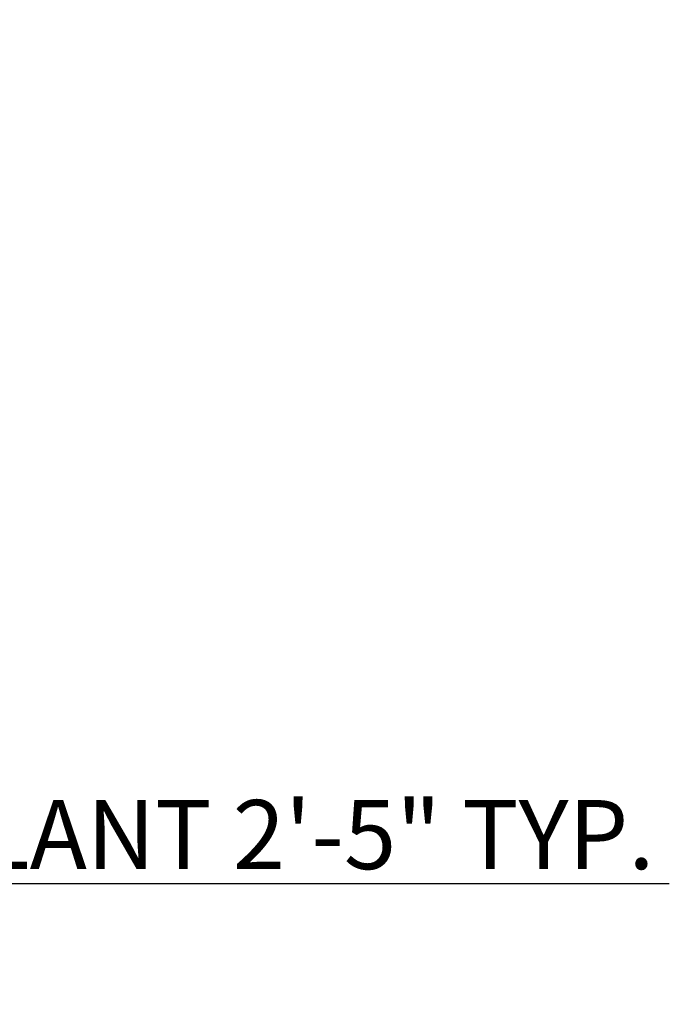
# Model space of a CAD drawing. Units: inches. Extents: x 3590 to 5167, y 65 to 1917.
# Tile 100 of 100: x 5082 to 5167, y 1747 to 1875. Entities that reach past the tile are written whole.
import ezdxf

# ---------------------------------------------------------------- set-up
doc = ezdxf.new("R2010")
doc.units = ezdxf.units.IN
doc.layers.add('A-ANNO-DIMS', color=2, linetype='Continuous', lineweight=18)
doc.styles.get("Standard").update_dxf_attribs({"font": 'arial.ttf'})
doc.dimstyles.new('ISO-25', dxfattribs={"dimtxt": 9, "dimasz": 2.5, "dimexe": 1.25, "dimexo": 0.625, "dimtad": 1, "dimdec": 1, "dimlunit": 3, "dimtxsty": 'Standard', "dimcen": 2.5, "dimadec": 0, "dimazin": 0, "dimtfac": 1, "dimtdec": 1, "dimtmove": 0, "dimatfit": 3, "dimfxl": 1, "dimarcsym": 0})

# ---------------------------------------------------------------- blocks, each defined once
blk = doc.blocks.new('*D322')
at = {"layer": 'A-ANNO-DIMS', "color": 0, "lineweight": -2, "transparency": 16777216}
for p, q in [((5035.74, 1766.18), (5035.74, 1761.2)), ((5064.81, 1766.18), (5064.81, 1761.2)), ((5038.24, 1762.45), (5062.31, 1762.45)), ((5064.81, 1762.45), (5166.99, 1762.45))]:
    blk.add_line(p, q, dxfattribs=at)
at = {"layer": 'A-ANNO-DIMS', "color": 0, "transparency": 16777216}
for points in [[(5038.24, 1762.87), (5038.24, 1762.03), (5035.74, 1762.45)], [(5062.31, 1762.87), (5062.31, 1762.03), (5064.81, 1762.45)]]:
    blk.add_solid(points, dxfattribs=at)
at = {"layer": 'Defpoints', "color": 0, "transparency": 16777216}
for p in [(5035.74, 1766.81), (5064.81, 1766.81), (5064.81, 1762.45)]:
    blk.add_point(p, dxfattribs=at)
at = {"layer": 'A-ANNO-DIMS', "color": 0, "transparency": 16777216, "insert": (5117.15, 1767.67), "char_height": 9, "attachment_point": 5}
blk.add_mtext('PLANT 2\'-5" TYP.', dxfattribs=at)
blk = doc.blocks.new('*D323')
at = {"layer": 'A-ANNO-DIMS', "color": 0, "lineweight": -2, "transparency": 16777216}
for p, q in [((5069.17, 1795.22), (5069.17, 1874.95)), ((5065.44, 1795.22), (5070.42, 1795.22)), ((5069.17, 1769.31), (5069.17, 1792.72)), ((5065.44, 1766.81), (5070.42, 1766.81))]:
    blk.add_line(p, q, dxfattribs=at)
at = {"layer": 'A-ANNO-DIMS', "color": 0, "transparency": 16777216}
for points in [[(5068.76, 1792.72), (5069.59, 1792.72), (5069.17, 1795.22)], [(5068.76, 1769.31), (5069.59, 1769.31), (5069.17, 1766.81)]]:
    blk.add_solid(points, dxfattribs=at)
at = {"layer": 'Defpoints', "color": 0, "transparency": 16777216}
for p in [(5064.81, 1795.22), (5069.17, 1795.22), (5064.81, 1766.81)]:
    blk.add_point(p, dxfattribs=at)
at = {"layer": 'A-ANNO-DIMS', "color": 0, "transparency": 16777216, "insert": (5063.89, 1836.33), "char_height": 9, "attachment_point": 5, "rotation": 90}
blk.add_mtext('2\'-4 1/2" TYP.', dxfattribs=at)

msp = doc.modelspace()

# ---------------------------------------------------------------- dimensions: what is measured, and where the dimension line sits
at = {"layer": 'A-ANNO-DIMS'}
dim = msp.add_linear_dim(base=(5069.17, 1795.22), p1=(5064.81, 1766.81), p2=(5064.81, 1795.22), angle=90, text='<> TYP.', dimstyle='ISO-25', override={"dimdec": 1, "dimlfac": 1, "dimrnd": 0, "dimzin": 1, "dimdsep": 46, "dimlunit": 4, "dimfrac": 2}, dxfattribs=at)
dim.commit()
dim.dimension.update_dxf_attribs({"geometry": '*D323', "text_midpoint": (5063.89, 1836.33)})
dim = msp.add_linear_dim(base=(5064.81, 1762.45), p1=(5035.74, 1766.81), p2=(5064.81, 1766.81), text='PLANT <> TYP.', dimstyle='ISO-25', override={"dimdec": 1, "dimlfac": 1, "dimrnd": 0, "dimzin": 1, "dimdsep": 46, "dimlunit": 4, "dimfrac": 2}, dxfattribs=at)
dim.commit()
dim.dimension.update_dxf_attribs({"geometry": '*D322', "text_midpoint": (5117.15, 1767.67)})

doc.saveas('drawing.dxf')
